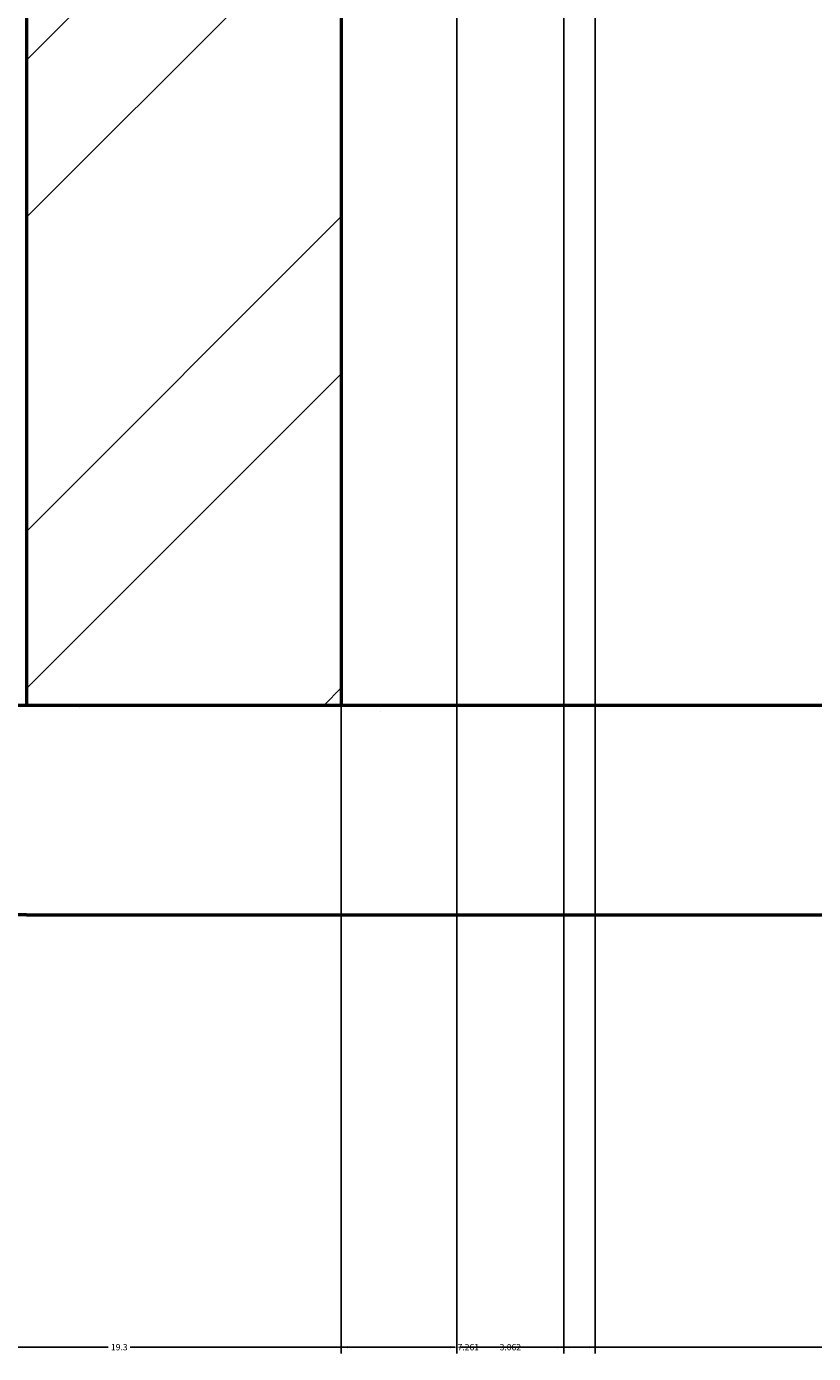
# Model space of a CAD drawing. Units: inches. Extents: x 2812 to 3051, y 1398 to 1659.
# Tile 2 of 65: x 2835 to 2858, y 1398 to 1435. Entities that reach past the tile are written whole.
import ezdxf

# ---------------------------------------------------------------- set-up
doc = ezdxf.new("R2010")
doc.units = ezdxf.units.IN
for name, color, linetype, lineweight in [('A-ANNO-DIMS', 2, 'Continuous', 18), ('S-CONC', 7, 'Continuous', 50), ('S-CONC-PATT', 8, 'Continuous', 18)]:
    doc.layers.add(name, color=color, linetype=linetype, lineweight=lineweight)
doc.styles.get("Standard").update_dxf_attribs({"font": 'arial.ttf'})
doc.dimstyles.get("Standard").update_dxf_attribs({"dimtxt": 0.18, "dimasz": 0.18, "dimexe": 0.18, "dimexo": 0.0625, "dimgap": 0.09, "dimtad": 0, "dimtih": 1, "dimtoh": 1, "dimdec": 4, "dimzin": 0, "dimdsep": 46, "dimtxsty": 'Standard', "dimcen": 0.09, "dimadec": 0, "dimazin": 0, "dimtfac": 1, "dimtdec": 4, "dimtofl": 0, "dimtmove": 0, "dimatfit": 3, "dimfxl": 1, "dimtolj": 1, "dimtzin": 0, "dimarcsym": 0})

# ---------------------------------------------------------------- blocks, each defined once
blk = doc.blocks.new('*D28')
at = {"layer": 'A-ANNO-DIMS', "color": 0, "lineweight": -2, "transparency": 16777216}
for p, q in [((2851.646, 1598.667), (2851.646, 1397.505)), ((2844.385, 1559.757), (2844.385, 1397.505)), ((2844.565, 1397.685), (2847.64, 1397.685)), ((2851.466, 1397.685), (2848.391, 1397.685))]:
    blk.add_line(p, q, dxfattribs=at)
at = {"layer": 'A-ANNO-DIMS', "color": 0, "transparency": 16777216}
for points in [[(2844.565, 1397.715), (2844.565, 1397.655), (2844.385, 1397.685)], [(2851.466, 1397.715), (2851.466, 1397.655), (2851.646, 1397.685)]]:
    blk.add_solid(points, dxfattribs=at)
at = {"layer": 'Defpoints', "color": 0, "transparency": 16777216}
for p in [(2851.646, 1598.73), (2844.385, 1559.82), (2851.646, 1397.685)]:
    blk.add_point(p, dxfattribs=at)
at = {"layer": 'A-ANNO-DIMS', "color": 0, "transparency": 16777216, "insert": (2848.016, 1397.685), "char_height": 0.18, "attachment_point": 5}
blk.add_mtext('\\A1;7.261', dxfattribs=at)
blk = doc.blocks.new('*D42')
at = {"layer": 'A-ANNO-DIMS', "color": 0, "lineweight": -2, "transparency": 16777216}
for p, q in [((2828.385, 1489.973), (2828.385, 1397.505)), ((2847.686, 1487.973), (2847.686, 1397.505)), ((2828.565, 1397.685), (2837.72, 1397.685)), ((2847.506, 1397.685), (2838.351, 1397.685))]:
    blk.add_line(p, q, dxfattribs=at)
at = {"layer": 'A-ANNO-DIMS', "color": 0, "transparency": 16777216}
for points in [[(2828.565, 1397.715), (2828.565, 1397.655), (2828.385, 1397.685)], [(2847.506, 1397.715), (2847.506, 1397.655), (2847.686, 1397.685)]]:
    blk.add_solid(points, dxfattribs=at)
at = {"layer": 'Defpoints', "color": 0, "transparency": 16777216}
for p in [(2828.385, 1490.035), (2847.686, 1488.035), (2847.686, 1397.685)]:
    blk.add_point(p, dxfattribs=at)
at = {"layer": 'A-ANNO-DIMS', "color": 0, "transparency": 16777216, "insert": (2838.036, 1397.685), "char_height": 0.18, "attachment_point": 5}
blk.add_mtext('\\A1;19.3', dxfattribs=at)
blk = doc.blocks.new('*D43')
at = {"layer": 'A-ANNO-DIMS', "color": 0, "lineweight": -2, "transparency": 16777216}
for p, q in [((2847.686, 1487.973), (2847.686, 1397.505)), ((2850.748, 1487.973), (2850.748, 1397.505)), ((2847.866, 1397.685), (2848.825, 1397.685)), ((2850.568, 1397.685), (2849.61, 1397.685))]:
    blk.add_line(p, q, dxfattribs=at)
at = {"layer": 'A-ANNO-DIMS', "color": 0, "transparency": 16777216}
for points in [[(2847.866, 1397.715), (2847.866, 1397.655), (2847.686, 1397.685)], [(2850.568, 1397.715), (2850.568, 1397.655), (2850.748, 1397.685)]]:
    blk.add_solid(points, dxfattribs=at)
at = {"layer": 'Defpoints', "color": 0, "transparency": 16777216}
for p in [(2847.686, 1488.035), (2850.748, 1488.035), (2850.748, 1397.685)]:
    blk.add_point(p, dxfattribs=at)
at = {"layer": 'A-ANNO-DIMS', "color": 0, "transparency": 16777216, "insert": (2849.217, 1397.685), "char_height": 0.18, "attachment_point": 5}
blk.add_mtext('\\A1;3.062', dxfattribs=at)
blk = doc.blocks.new('*D44')
at = {"layer": 'A-ANNO-DIMS', "color": 0, "lineweight": -2, "transparency": 16777216}
for p, q in [((2850.748, 1487.973), (2850.748, 1397.505)), ((2896.385, 1487.973), (2896.385, 1397.505)), ((2850.928, 1397.685), (2873.17, 1397.685)), ((2896.205, 1397.685), (2873.964, 1397.685))]:
    blk.add_line(p, q, dxfattribs=at)
at = {"layer": 'A-ANNO-DIMS', "color": 0, "transparency": 16777216}
for points in [[(2850.928, 1397.715), (2850.928, 1397.655), (2850.748, 1397.685)], [(2896.205, 1397.715), (2896.205, 1397.655), (2896.385, 1397.685)]]:
    blk.add_solid(points, dxfattribs=at)
at = {"layer": 'Defpoints', "color": 0, "transparency": 16777216}
for p in [(2850.748, 1488.035), (2896.385, 1488.035), (2896.385, 1397.685)]:
    blk.add_point(p, dxfattribs=at)
at = {"layer": 'A-ANNO-DIMS', "color": 0, "transparency": 16777216, "insert": (2873.567, 1397.685), "char_height": 0.18, "attachment_point": 5}
blk.add_mtext('\\A1;45.64', dxfattribs=at)
blk = doc.blocks.new('*D56')
at = {"layer": 'A-ANNO-DIMS', "color": 0, "lineweight": -2, "transparency": 16777216}
for p, q in [((2880.322, 1452.035), (2811.806, 1452.035)), ((2811.986, 1451.855), (2811.986, 1434.217)), ((2811.986, 1416.215), (2811.986, 1433.853)), ((2952.322, 1416.035), (2811.806, 1416.035))]:
    blk.add_line(p, q, dxfattribs=at)
at = {"layer": 'A-ANNO-DIMS', "color": 0, "transparency": 16777216}
for points in [[(2811.956, 1451.855), (2812.016, 1451.855), (2811.986, 1452.035)], [(2811.956, 1416.215), (2812.016, 1416.215), (2811.986, 1416.035)]]:
    blk.add_solid(points, dxfattribs=at)
at = {"layer": 'Defpoints', "color": 0, "transparency": 16777216}
for p in [(2811.986, 1452.035), (2880.385, 1452.035), (2952.385, 1416.035)]:
    blk.add_point(p, dxfattribs=at)
at = {"layer": 'A-ANNO-DIMS', "color": 0, "transparency": 16777216, "insert": (2811.986, 1434.035), "char_height": 0.18, "attachment_point": 5}
blk.add_mtext('\\A1;36', dxfattribs=at)
blk = doc.blocks.new('*D75')
at = {"layer": 'A-ANNO-DIMS', "color": 0, "lineweight": -2, "transparency": 16777216}
for p, q in [((2963.812, 1448.474), (2811.806, 1448.474)), ((2811.986, 1448.294), (2811.986, 1432.437)), ((2811.986, 1416.215), (2811.986, 1432.073)), ((2961.322, 1416.035), (2811.806, 1416.035))]:
    blk.add_line(p, q, dxfattribs=at)
at = {"layer": 'A-ANNO-DIMS', "color": 0, "transparency": 16777216}
for points in [[(2811.956, 1448.294), (2812.016, 1448.294), (2811.986, 1448.474)], [(2811.956, 1416.215), (2812.016, 1416.215), (2811.986, 1416.035)]]:
    blk.add_solid(points, dxfattribs=at)
at = {"layer": 'Defpoints', "color": 0, "transparency": 16777216}
for p in [(2811.986, 1448.474), (2963.874, 1448.474), (2961.385, 1416.035)]:
    blk.add_point(p, dxfattribs=at)
at = {"layer": 'A-ANNO-DIMS', "color": 0, "transparency": 16777216, "insert": (2811.986, 1432.255), "char_height": 0.18, "attachment_point": 5}
blk.add_mtext('\\A1;32.44', dxfattribs=at)

msp = doc.modelspace()

# ---------------------------------------------------------------- hatches: boundary and pattern name
at = {"layer": 'S-CONC-PATT'}
h = msp.add_hatch(dxfattribs=at)
h.set_pattern_fill('ANSI32', color=256)
h.paths.add_polyline_path([(3027.3849, 1646.82), (2835.3849, 1646.82), (2835.3849, 1603.2296), (2844.3849, 1603.2296), (2844.3849, 1637.82), (3018.3849, 1637.82), (3018.3849, 1602.5441), (3027.3849, 1602.5441)])
h.paths.add_polyline_path([(2844.3849, 1594.2296), (2835.3849, 1594.2296), (2835.3849, 1550.82), (3027.3849, 1550.82), (3027.3849, 1593.5441), (3018.3849, 1593.5441), (3018.3849, 1559.82), (2844.3849, 1559.82)])
h.paths.add_polyline_path([(2844.3849, 1482.0354), (2835.3849, 1482.0354), (2835.3849, 1463.4959), (2844.3849, 1463.4959)])
h.paths.add_polyline_path([(2844.3849, 1461.4959), (2835.3849, 1461.4959), (2835.3849, 1416.0354), (2844.3849, 1416.0354)])
h.paths.add_polyline_path([(3027.3849, 1482.0354), (3018.3849, 1482.0354), (3018.3849, 1463.2854), (3027.3849, 1463.2854)])
h.paths.add_polyline_path([(3027.3849, 1461.2854), (3018.3849, 1461.2854), (3018.3849, 1416.0354), (3027.3849, 1416.0354)])
h.paths.add_polyline_path([(2961.3849, 1448.4738), (2952.3849, 1448.4738), (2952.3849, 1416.0354), (2961.3849, 1416.0354)])
h.paths.add_polyline_path([(2961.3849, 1462.3026), (2952.3849, 1462.3026), (2952.3849, 1450.4738), (2961.3849, 1450.4738)])
h.paths.add_polyline_path([(2961.3849, 1472.0354), (2952.3849, 1472.0354), (2952.3849, 1462.3026), (2961.3849, 1462.3026)])
h = msp.add_hatch(dxfattribs=at)
h.set_pattern_fill('AR-SAND', color=256, scale=0.3)
h.paths.add_polyline_path([(3036.3849, 1416.0354), (3027.3849, 1416.0354), (2826.3849, 1416.0354), (2826.3849, 1410.0354), (2835.3849, 1410.0354), (3036.3849, 1410.0354)])
h.paths.add_polyline_path([(2970.3849, 1488.0354), (2969.3849, 1488.0354), (2941.3849, 1488.0354), (2941.3849, 1482.0354), (2970.3849, 1482.0354)])
h.paths.add_polyline_path([(3036.3849, 1488.0354), (3035.3849, 1488.0354), (3006.3849, 1488.0354), (3006.3849, 1482.0354), (3027.3849, 1482.0354), (3036.3849, 1482.0354)])
h.paths.add_polyline_path([(3034.3849, 1490.0354), (3008.3849, 1490.0354), (3008.3849, 1489.0354), (3034.3849, 1489.0354)])
h.paths.add_polyline_path([(3035.3849, 1489.0354), (3034.3849, 1489.0354), (3007.3849, 1489.0354), (3007.3849, 1488.0354), (3035.3849, 1488.0354)])
h.paths.add_polyline_path([(2968.3849, 1490.0354), (2943.3849, 1490.0354), (2943.3849, 1489.0354), (2968.3849, 1489.0354)])
h.paths.add_polyline_path([(2969.3849, 1489.0354), (2968.3849, 1489.0354), (2942.3849, 1489.0354), (2942.3849, 1488.0354), (2969.3849, 1488.0354)])
h.paths.add_polyline_path([(2896.3849, 1488.0354), (2826.3849, 1488.0354), (2826.3849, 1482.0354), (2896.3849, 1482.0354)])
h.paths.add_polyline_path([(2895.3849, 1489.0354), (2894.3849, 1489.0354), (2827.3849, 1489.0354), (2827.3849, 1488.0354), (2895.3849, 1488.0354)])
h.paths.add_polyline_path([(2894.3849, 1490.0354), (2828.3849, 1490.0354), (2828.3849, 1489.0354), (2894.3849, 1489.0354)])
h = msp.add_hatch(dxfattribs=at)
h.set_pattern_fill('AR-CONC', color=256, scale=0.3)
h.paths.add_polyline_path([(3036.3849, 1416.0354), (3027.3849, 1416.0354), (2826.3849, 1416.0354), (2826.3849, 1410.0354), (2835.3849, 1410.0354), (3036.3849, 1410.0354)])

# ---------------------------------------------------------------- linework, layer by layer
at = {"layer": 'S-CONC'}
for p, q in [((2835.3849, 1482.0354), (2835.3849, 1416.0354)), ((2835.3849, 1482.0354), (2835.3849, 1416.0354)), ((2844.3849, 1482.0354), (2844.3849, 1416.0354)), ((2826.3849, 1416.0354), (3027.3849, 1416.0354)), ((2835.3849, 1410.0354), (2826.3849, 1410.0354)), ((2835.3849, 1410.0354), (3036.3849, 1410.0354))]:
    msp.add_line(p, q, dxfattribs=at)

# ---------------------------------------------------------------- dimensions: what is measured, and where the dimension line sits
at = {"layer": 'A-ANNO-DIMS'}
for base, p1, p2, override, picture, middle in [((2851.6462, 1397.6854), (2844.3849, 1559.82), (2851.6462, 1598.7296), {"dimdec": 3, "dimlfac": 1, "dimrnd": 0, "dimzin": 0, "dimdsep": 46, "dimlunit": 2}, '*D28', (2848.0156, 1397.6854)), ((2847.6863, 1397.6854), (2828.3849, 1490.0354), (2847.6863, 1488.0354), {"dimdec": 1, "dimlfac": 1, "dimrnd": 0, "dimzin": 0, "dimdsep": 46, "dimlunit": 2}, '*D42', (2838.0356, 1397.6854)), ((2850.7485, 1397.6854), (2847.6863, 1488.0354), (2850.7485, 1488.0354), {"dimdec": 3, "dimlfac": 1, "dimrnd": 0, "dimzin": 0, "dimdsep": 46, "dimlunit": 2}, '*D43', (2849.2174, 1397.6854)), ((2896.3849, 1397.6854), (2850.7485, 1488.0354), (2896.3849, 1488.0354), {"dimdec": 2, "dimlfac": 1, "dimrnd": 0, "dimzin": 0, "dimdsep": 46, "dimlunit": 2}, '*D44', (2873.5667, 1397.6854))]:
    dim = msp.add_linear_dim(base=base, p1=p1, p2=p2, dimstyle='Standard', override=override, dxfattribs=at)
    dim.commit()
    dim.dimension.update_dxf_attribs({"geometry": picture, "text_midpoint": middle})
for base, p1, p2, override, picture, middle in [((2811.9855, 1452.0354), (2952.3849, 1416.0354), (2880.3849, 1452.0354), {"dimdec": 0, "dimlfac": 1, "dimrnd": 0, "dimzin": 0, "dimdsep": 46, "dimlunit": 2}, '*D56', (2811.9855, 1434.0354)), ((2811.9855, 1448.4738), (2961.3849, 1416.0354), (2963.8741, 1448.4738), {"dimdec": 2, "dimlfac": 1, "dimrnd": 0, "dimzin": 0, "dimdsep": 46, "dimlunit": 2}, '*D75', (2811.9855, 1432.2546))]:
    dim = msp.add_linear_dim(base=base, p1=p1, p2=p2, angle=90, dimstyle='Standard', override=override, dxfattribs=at)
    dim.commit()
    dim.dimension.update_dxf_attribs({"geometry": picture, "text_midpoint": middle})

doc.saveas('drawing.dxf')
